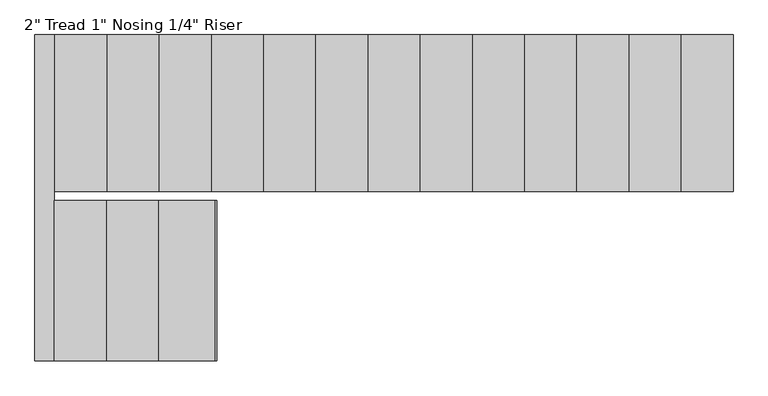
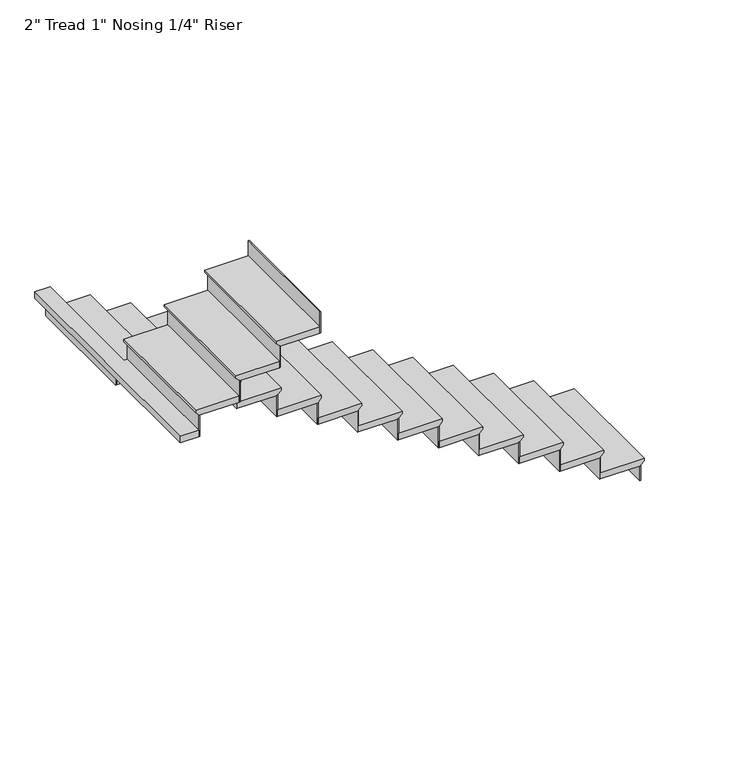
"""IFC4 building model written with IfcOpenShell, lengths in millimetres: stair flight geometry."""

from ifc_helpers import new_model, si_unit, origin, place, context, project, spatial, faceted_brep, source, transform, mapped, element, save


def stair_flight_dace13c7(model_context):
    return source(origin(), model_context, "Body", "Brep", [
        faceted_brep([(6794.5, 11386.0372886, 3198.2833333), (6794.5, 11386.0372886, 3217.3333333), (6794.5, 10471.6372886, 3217.3333333), (6794.5, 10471.6372886, 3198.2833333), (6769.1, 11386.0372886, 3172.8833333), (6769.1, 10471.6372886, 3172.8833333), (6464.3, 11386.0372886, 3217.3333333), (6464.3, 10471.6372886, 3217.3333333), (6769.1, 10471.6372886, 3166.5333333), (6464.3, 10471.6372886, 3166.5333333), (6464.3, 11386.0372886, 3166.5333333), (6769.1, 11386.0372886, 3166.5333333)], [[[0, 1, 2, 3]], [[4, 0, 3, 5]], [[2, 1, 6, 7]], [[8, 9, 10, 11]], [[2, 7, 9, 8, 5, 3]], [[8, 11, 4, 5]], [[6, 1, 0, 4, 11, 10]], [[7, 6, 10, 9]]]),
        faceted_brep([(6769.1, 11386.0372886, 3166.5333333), (6769.1, 11386.0372886, 3048.0), (6762.75, 11386.0372886, 3048.0), (6762.75, 11386.0372886, 3166.5333333), (6769.1, 10471.6372886, 3166.5333333), (6762.75, 10471.6372886, 3166.5333333), (6762.75, 10471.6372886, 3048.0), (6769.1, 10471.6372886, 3048.0)], [[[0, 1, 2, 3]], [[4, 5, 6, 7]], [[1, 0, 4, 7]], [[2, 1, 7, 6]], [[3, 2, 6, 5]], [[0, 3, 5, 4]]]),
        faceted_brep([(6464.3, 11386.0372886, 3335.8666667), (6464.3, 11386.0372886, 3166.5333333), (6457.95, 11386.0372886, 3166.5333333), (6457.95, 11386.0372886, 3335.8666667), (6464.3, 10471.6372886, 3335.8666667), (6457.95, 10471.6372886, 3335.8666667), (6457.95, 10471.6372886, 3166.5333333), (6464.3, 10471.6372886, 3166.5333333)], [[[0, 1, 2, 3]], [[4, 5, 6, 7]], [[1, 0, 4, 7]], [[2, 1, 7, 6]], [[3, 2, 6, 5]], [[0, 3, 5, 4]]]),
        faceted_brep([(6489.7, 10471.6372886, 3386.6666667), (6489.7, 11386.0372886, 3386.6666667), (6159.5, 11386.0372886, 3386.6666667), (6159.5, 10471.6372886, 3386.6666667), (6464.3, 10471.6372886, 3335.8666667), (6159.5, 10471.6372886, 3335.8666667), (6159.5, 11386.0372886, 3335.8666667), (6464.3, 11386.0372886, 3335.8666667), (6464.3, 10471.6372886, 3342.2166667), (6489.7, 10471.6372886, 3367.6166667), (6464.3, 11386.0372886, 3342.2166667), (6489.7, 11386.0372886, 3367.6166667)], [[[0, 1, 2, 3]], [[4, 5, 6, 7]], [[0, 3, 5, 4, 8, 9]], [[4, 7, 10, 8]], [[2, 1, 11, 10, 7, 6]], [[3, 2, 6, 5]], [[11, 1, 0, 9]], [[10, 11, 9, 8]]]),
        faceted_brep([(6159.5, 11386.0372886, 3505.2), (6159.5, 11386.0372886, 3335.8666667), (6153.15, 11386.0372886, 3335.8666667), (6153.15, 11386.0372886, 3505.2), (6159.5, 10471.6372886, 3505.2), (6153.15, 10471.6372886, 3505.2), (6153.15, 10471.6372886, 3335.8666667), (6159.5, 10471.6372886, 3335.8666667)], [[[0, 1, 2, 3]], [[4, 5, 6, 7]], [[1, 0, 4, 7]], [[2, 1, 7, 6]], [[3, 2, 6, 5]], [[0, 3, 5, 4]]]),
        faceted_brep([(6184.9, 10471.6372886, 3556.0), (6184.9, 11386.0372886, 3556.0), (5854.7, 11386.0372886, 3556.0), (5854.7, 10471.6372886, 3556.0), (6159.5, 10471.6372886, 3505.2), (5854.7, 10471.6372886, 3505.2), (5854.7, 11386.0372886, 3505.2), (6159.5, 11386.0372886, 3505.2), (6159.5, 10471.6372886, 3511.55), (6184.9, 10471.6372886, 3536.95), (6159.5, 11386.0372886, 3511.55), (6184.9, 11386.0372886, 3536.95)], [[[0, 1, 2, 3]], [[4, 5, 6, 7]], [[0, 3, 5, 4, 8, 9]], [[4, 7, 10, 8]], [[2, 1, 11, 10, 7, 6]], [[3, 2, 6, 5]], [[11, 1, 0, 9]], [[10, 11, 9, 8]]]),
        faceted_brep([(5854.7, 11386.0372886, 3674.5333333), (5854.7, 11386.0372886, 3505.2), (5848.35, 11386.0372886, 3505.2), (5848.35, 11386.0372886, 3674.5333333), (5854.7, 10471.6372886, 3674.5333333), (5848.35, 10471.6372886, 3674.5333333), (5848.35, 10471.6372886, 3505.2), (5854.7, 10471.6372886, 3505.2)], [[[0, 1, 2, 3]], [[4, 5, 6, 7]], [[1, 0, 4, 7]], [[2, 1, 7, 6]], [[3, 2, 6, 5]], [[0, 3, 5, 4]]]),
        faceted_brep([(5880.1, 10471.6372886, 3725.3333333), (5880.1, 11386.0372886, 3725.3333333), (5549.9, 11386.0372886, 3725.3333333), (5549.9, 10471.6372886, 3725.3333333), (5854.7, 10471.6372886, 3674.5333333), (5549.9, 10471.6372886, 3674.5333333), (5549.9, 11386.0372886, 3674.5333333), (5854.7, 11386.0372886, 3674.5333333), (5854.7, 10471.6372886, 3680.8833333), (5880.1, 10471.6372886, 3706.2833333), (5854.7, 11386.0372886, 3680.8833333), (5880.1, 11386.0372886, 3706.2833333)], [[[0, 1, 2, 3]], [[4, 5, 6, 7]], [[0, 3, 5, 4, 8, 9]], [[4, 7, 10, 8]], [[2, 1, 11, 10, 7, 6]], [[3, 2, 6, 5]], [[11, 1, 0, 9]], [[10, 11, 9, 8]]]),
        faceted_brep([(5549.9, 11386.0372886, 3843.8666667), (5549.9, 11386.0372886, 3674.5333333), (5543.55, 11386.0372886, 3674.5333333), (5543.55, 11386.0372886, 3843.8666667), (5549.9, 10471.6372886, 3843.8666667), (5543.55, 10471.6372886, 3843.8666667), (5543.55, 10471.6372886, 3674.5333333), (5549.9, 10471.6372886, 3674.5333333)], [[[0, 1, 2, 3]], [[4, 5, 6, 7]], [[1, 0, 4, 7]], [[2, 1, 7, 6]], [[3, 2, 6, 5]], [[0, 3, 5, 4]]]),
        faceted_brep([(5575.3, 10471.6372886, 3894.6666667), (5575.3, 11386.0372886, 3894.6666667), (5245.1, 11386.0372886, 3894.6666667), (5245.1, 10471.6372886, 3894.6666667), (5549.9, 10471.6372886, 3843.8666667), (5245.1, 10471.6372886, 3843.8666667), (5245.1, 11386.0372886, 3843.8666667), (5549.9, 11386.0372886, 3843.8666667), (5549.9, 10471.6372886, 3850.2166667), (5575.3, 10471.6372886, 3875.6166667), (5549.9, 11386.0372886, 3850.2166667), (5575.3, 11386.0372886, 3875.6166667)], [[[0, 1, 2, 3]], [[4, 5, 6, 7]], [[0, 3, 5, 4, 8, 9]], [[4, 7, 10, 8]], [[2, 1, 11, 10, 7, 6]], [[3, 2, 6, 5]], [[11, 1, 0, 9]], [[10, 11, 9, 8]]]),
        faceted_brep([(5245.1, 11386.0372886, 4013.2), (5245.1, 11386.0372886, 3843.8666667), (5238.75, 11386.0372886, 3843.8666667), (5238.75, 11386.0372886, 4013.2), (5245.1, 10471.6372886, 4013.2), (5238.75, 10471.6372886, 4013.2), (5238.75, 10471.6372886, 3843.8666667), (5245.1, 10471.6372886, 3843.8666667)], [[[0, 1, 2, 3]], [[4, 5, 6, 7]], [[1, 0, 4, 7]], [[2, 1, 7, 6]], [[3, 2, 6, 5]], [[0, 3, 5, 4]]]),
        faceted_brep([(5270.5, 10471.6372886, 4064.0), (5270.5, 11386.0372886, 4064.0), (4940.3, 11386.0372886, 4064.0), (4940.3, 10471.6372886, 4064.0), (5245.1, 10471.6372886, 4013.2), (4940.3, 10471.6372886, 4013.2), (4940.3, 11386.0372886, 4013.2), (5245.1, 11386.0372886, 4013.2), (5245.1, 10471.6372886, 4019.55), (5270.5, 10471.6372886, 4044.95), (5245.1, 11386.0372886, 4019.55), (5270.5, 11386.0372886, 4044.95)], [[[0, 1, 2, 3]], [[4, 5, 6, 7]], [[0, 3, 5, 4, 8, 9]], [[4, 7, 10, 8]], [[2, 1, 11, 10, 7, 6]], [[3, 2, 6, 5]], [[11, 1, 0, 9]], [[10, 11, 9, 8]]]),
        faceted_brep([(4940.3, 11386.0372886, 4182.5333333), (4940.3, 11386.0372886, 4013.2), (4933.95, 11386.0372886, 4013.2), (4933.95, 11386.0372886, 4182.5333333), (4940.3, 10471.6372886, 4182.5333333), (4933.95, 10471.6372886, 4182.5333333), (4933.95, 10471.6372886, 4013.2), (4940.3, 10471.6372886, 4013.2)], [[[0, 1, 2, 3]], [[4, 5, 6, 7]], [[1, 0, 4, 7]], [[2, 1, 7, 6]], [[3, 2, 6, 5]], [[0, 3, 5, 4]]]),
        faceted_brep([(4965.7, 10471.6372886, 4233.3333333), (4965.7, 11386.0372886, 4233.3333333), (4635.5, 11386.0372886, 4233.3333333), (4635.5, 10471.6372886, 4233.3333333), (4940.3, 10471.6372886, 4182.5333333), (4635.5, 10471.6372886, 4182.5333333), (4635.5, 11386.0372886, 4182.5333333), (4940.3, 11386.0372886, 4182.5333333), (4940.3, 10471.6372886, 4188.8833333), (4965.7, 10471.6372886, 4214.2833333), (4940.3, 11386.0372886, 4188.8833333), (4965.7, 11386.0372886, 4214.2833333)], [[[0, 1, 2, 3]], [[4, 5, 6, 7]], [[0, 3, 5, 4, 8, 9]], [[4, 7, 10, 8]], [[2, 1, 11, 10, 7, 6]], [[3, 2, 6, 5]], [[11, 1, 0, 9]], [[10, 11, 9, 8]]]),
        faceted_brep([(4635.5, 11386.0372886, 4351.8666667), (4635.5, 11386.0372886, 4182.5333333), (4629.15, 11386.0372886, 4182.5333333), (4629.15, 11386.0372886, 4351.8666667), (4635.5, 10471.6372886, 4351.8666667), (4629.15, 10471.6372886, 4351.8666667), (4629.15, 10471.6372886, 4182.5333333), (4635.5, 10471.6372886, 4182.5333333)], [[[0, 1, 2, 3]], [[4, 5, 6, 7]], [[1, 0, 4, 7]], [[2, 1, 7, 6]], [[3, 2, 6, 5]], [[0, 3, 5, 4]]]),
        faceted_brep([(4660.9, 10471.6372886, 4402.6666667), (4660.9, 11386.0372886, 4402.6666667), (4330.7, 11386.0372886, 4402.6666667), (4330.7, 10471.6372886, 4402.6666667), (4635.5, 10471.6372886, 4351.8666667), (4330.7, 10471.6372886, 4351.8666667), (4330.7, 11386.0372886, 4351.8666667), (4635.5, 11386.0372886, 4351.8666667), (4635.5, 10471.6372886, 4358.2166667), (4660.9, 10471.6372886, 4383.6166667), (4635.5, 11386.0372886, 4358.2166667), (4660.9, 11386.0372886, 4383.6166667)], [[[0, 1, 2, 3]], [[4, 5, 6, 7]], [[0, 3, 5, 4, 8, 9]], [[4, 7, 10, 8]], [[2, 1, 11, 10, 7, 6]], [[3, 2, 6, 5]], [[11, 1, 0, 9]], [[10, 11, 9, 8]]]),
        faceted_brep([(4330.7, 11386.0372886, 4521.2), (4330.7, 11386.0372886, 4351.8666667), (4324.35, 11386.0372886, 4351.8666667), (4324.35, 11386.0372886, 4521.2), (4330.7, 10471.6372886, 4521.2), (4324.35, 10471.6372886, 4521.2), (4324.35, 10471.6372886, 4351.8666667), (4330.7, 10471.6372886, 4351.8666667)], [[[0, 1, 2, 3]], [[4, 5, 6, 7]], [[1, 0, 4, 7]], [[2, 1, 7, 6]], [[3, 2, 6, 5]], [[0, 3, 5, 4]]]),
        faceted_brep([(4356.1, 10471.6372886, 4572.0), (4356.1, 11386.0372886, 4572.0), (4025.9, 11386.0372886, 4572.0), (4025.9, 10471.6372886, 4572.0), (4330.7, 10471.6372886, 4521.2), (4025.9, 10471.6372886, 4521.2), (4025.9, 11386.0372886, 4521.2), (4330.7, 11386.0372886, 4521.2), (4330.7, 10471.6372886, 4527.55), (4356.1, 10471.6372886, 4552.95), (4330.7, 11386.0372886, 4527.55), (4356.1, 11386.0372886, 4552.95)], [[[0, 1, 2, 3]], [[4, 5, 6, 7]], [[0, 3, 5, 4, 8, 9]], [[4, 7, 10, 8]], [[2, 1, 11, 10, 7, 6]], [[3, 2, 6, 5]], [[11, 1, 0, 9]], [[10, 11, 9, 8]]]),
        faceted_brep([(4025.9, 11386.0372886, 4690.5333333), (4025.9, 11386.0372886, 4521.2), (4019.55, 11386.0372886, 4521.2), (4019.55, 11386.0372886, 4690.5333333), (4025.9, 10471.6372886, 4690.5333333), (4019.55, 10471.6372886, 4690.5333333), (4019.55, 10471.6372886, 4521.2), (4025.9, 10471.6372886, 4521.2)], [[[0, 1, 2, 3]], [[4, 5, 6, 7]], [[1, 0, 4, 7]], [[2, 1, 7, 6]], [[3, 2, 6, 5]], [[0, 3, 5, 4]]]),
        faceted_brep([(4051.3, 10471.6372886, 4741.3333333), (4051.3, 11386.0372886, 4741.3333333), (3721.1, 11386.0372886, 4741.3333333), (3721.1, 10471.6372886, 4741.3333333), (4025.9, 10471.6372886, 4690.5333333), (3721.1, 10471.6372886, 4690.5333333), (3721.1, 11386.0372886, 4690.5333333), (4025.9, 11386.0372886, 4690.5333333), (4025.9, 10471.6372886, 4696.8833333), (4051.3, 10471.6372886, 4722.2833333), (4025.9, 11386.0372886, 4696.8833333), (4051.3, 11386.0372886, 4722.2833333)], [[[0, 1, 2, 3]], [[4, 5, 6, 7]], [[0, 3, 5, 4, 8, 9]], [[4, 7, 10, 8]], [[2, 1, 11, 10, 7, 6]], [[3, 2, 6, 5]], [[11, 1, 0, 9]], [[10, 11, 9, 8]]]),
        faceted_brep([(3721.1, 11386.0372886, 4859.8666667), (3721.1, 11386.0372886, 4690.5333333), (3714.75, 11386.0372886, 4690.5333333), (3714.75, 11386.0372886, 4859.8666667), (3721.1, 10471.6372886, 4859.8666667), (3714.75, 10471.6372886, 4859.8666667), (3714.75, 10471.6372886, 4690.5333333), (3721.1, 10471.6372886, 4690.5333333)], [[[0, 1, 2, 3]], [[4, 5, 6, 7]], [[1, 0, 4, 7]], [[2, 1, 7, 6]], [[3, 2, 6, 5]], [[0, 3, 5, 4]]]),
        faceted_brep([(3746.5, 10471.6372886, 4910.6666667), (3746.5, 11386.0372886, 4910.6666667), (3416.3, 11386.0372886, 4910.6666667), (3416.3, 10471.6372886, 4910.6666667), (3721.1, 10471.6372886, 4859.8666667), (3416.3, 10471.6372886, 4859.8666667), (3416.3, 11386.0372886, 4859.8666667), (3721.1, 11386.0372886, 4859.8666667), (3721.1, 10471.6372886, 4866.2166667), (3746.5, 10471.6372886, 4891.6166667), (3721.1, 11386.0372886, 4866.2166667), (3746.5, 11386.0372886, 4891.6166667)], [[[0, 1, 2, 3]], [[4, 5, 6, 7]], [[0, 3, 5, 4, 8, 9]], [[4, 7, 10, 8]], [[2, 1, 11, 10, 7, 6]], [[3, 2, 6, 5]], [[11, 1, 0, 9]], [[10, 11, 9, 8]]]),
        faceted_brep([(3416.3, 11386.0372886, 5029.2), (3416.3, 11386.0372886, 4859.8666667), (3409.95, 11386.0372886, 4859.8666667), (3409.95, 11386.0372886, 5029.2), (3416.3, 10471.6372886, 5029.2), (3409.95, 10471.6372886, 5029.2), (3409.95, 10471.6372886, 4859.8666667), (3416.3, 10471.6372886, 4859.8666667)], [[[0, 1, 2, 3]], [[4, 5, 6, 7]], [[1, 0, 4, 7]], [[2, 1, 7, 6]], [[3, 2, 6, 5]], [[0, 3, 5, 4]]]),
        faceted_brep([(3441.7, 10471.6372886, 5080.0), (3441.7, 11386.0372886, 5080.0), (3111.5, 11386.0372886, 5080.0), (3111.5, 10471.6372886, 5080.0), (3416.3, 10471.6372886, 5029.2), (3111.5, 10471.6372886, 5029.2), (3111.5, 11386.0372886, 5029.2), (3416.3, 11386.0372886, 5029.2), (3416.3, 10471.6372886, 5035.55), (3441.7, 10471.6372886, 5060.95), (3416.3, 11386.0372886, 5035.55), (3441.7, 11386.0372886, 5060.95)], [[[0, 1, 2, 3]], [[4, 5, 6, 7]], [[0, 3, 5, 4, 8, 9]], [[4, 7, 10, 8]], [[2, 1, 11, 10, 7, 6]], [[3, 2, 6, 5]], [[11, 1, 0, 9]], [[10, 11, 9, 8]]]),
        faceted_brep([(3111.5, 11386.0372886, 5198.5333333), (3111.5, 11386.0372886, 5029.2), (3105.15, 11386.0372886, 5029.2), (3105.15, 11386.0372886, 5198.5333333), (3111.5, 10471.6372886, 5198.5333333), (3105.15, 10471.6372886, 5198.5333333), (3105.15, 10471.6372886, 5029.2), (3111.5, 10471.6372886, 5029.2)], [[[0, 1, 2, 3]], [[4, 5, 6, 7]], [[1, 0, 4, 7]], [[2, 1, 7, 6]], [[3, 2, 6, 5]], [[0, 3, 5, 4]]]),
        faceted_brep([(3136.9, 10471.6372886, 5249.3333333), (3136.9, 11386.0372886, 5249.3333333), (2806.7, 11386.0372886, 5249.3333333), (2806.7, 10471.6372886, 5249.3333333), (3111.5, 10471.6372886, 5198.5333333), (2806.7, 10471.6372886, 5198.5333333), (2806.7, 11386.0372886, 5198.5333333), (3111.5, 11386.0372886, 5198.5333333), (3111.5, 10471.6372886, 5204.8833333), (3136.9, 10471.6372886, 5230.2833333), (3111.5, 11386.0372886, 5204.8833333), (3136.9, 11386.0372886, 5230.2833333)], [[[0, 1, 2, 3]], [[4, 5, 6, 7]], [[0, 3, 5, 4, 8, 9]], [[4, 7, 10, 8]], [[2, 1, 11, 10, 7, 6]], [[3, 2, 6, 5]], [[11, 1, 0, 9]], [[10, 11, 9, 8]]]),
        faceted_brep([(2806.7, 11386.0372886, 5367.8666667), (2806.7, 11386.0372886, 5198.5333333), (2800.35, 11386.0372886, 5198.5333333), (2800.35, 11386.0372886, 5367.8666667), (2806.7, 10471.6372886, 5367.8666667), (2800.35, 10471.6372886, 5367.8666667), (2800.35, 10471.6372886, 5198.5333333), (2806.7, 10471.6372886, 5198.5333333)], [[[0, 1, 2, 3]], [[4, 5, 6, 7]], [[1, 0, 4, 7]], [[2, 1, 7, 6]], [[3, 2, 6, 5]], [[0, 3, 5, 4]]]),
        faceted_brep([(2857.5, 10418.2972886, 5418.6666667), (2832.1, 10418.2972886, 5418.6666667), (2832.1, 11386.0372886, 5418.6666667), (2717.8, 11386.0372886, 5418.6666667), (2717.8, 9481.0372886, 5418.6666667), (2857.5, 9481.0372886, 5418.6666667), (2832.1, 10418.2972886, 5367.8666667), (2857.5, 10418.2972886, 5367.8666667), (2857.5, 9481.0372886, 5367.8666667), (2717.8, 9481.0372886, 5367.8666667), (2717.8, 11386.0372886, 5367.8666667), (2806.7, 11386.0372886, 5367.8666667), (2806.7, 10471.6372886, 5367.8666667), (2832.1, 10471.6372886, 5367.8666667), (2832.1, 10471.6372886, 5399.6166667), (2832.1, 11386.0372886, 5399.6166667), (2806.7, 10471.6372886, 5374.2166667), (2806.7, 11386.0372886, 5374.2166667)], [[[0, 1, 2, 3, 4, 5]], [[6, 7, 8, 9, 10, 11, 12, 13]], [[1, 0, 7, 6]], [[2, 1, 6, 13, 14, 15]], [[13, 12, 16, 14]], [[12, 11, 17, 16]], [[3, 2, 15, 17, 11, 10]], [[4, 3, 10, 9]], [[5, 4, 9, 8]], [[0, 5, 8, 7]], [[17, 15, 14, 16]]]),
        faceted_brep([(2857.5, 9481.0372886, 5537.2), (2857.5, 9481.0372886, 5367.8666667), (2863.85, 9481.0372886, 5367.8666667), (2863.85, 9481.0372886, 5537.2), (2857.5, 10418.2972886, 5537.2), (2863.85, 10418.2972886, 5537.2), (2863.85, 10418.2972886, 5367.8666667), (2857.5, 10418.2972886, 5367.8666667)], [[[0, 1, 2, 3]], [[4, 5, 6, 7]], [[1, 0, 4, 7]], [[2, 1, 7, 6]], [[3, 2, 6, 5]], [[0, 3, 5, 4]]]),
        faceted_brep([(2832.1, 10418.2972886, 5588.0), (2832.1, 9481.0372886, 5588.0), (3162.3, 9481.0372886, 5588.0), (3162.3, 10418.2972886, 5588.0), (2857.5, 10418.2972886, 5537.2), (3162.3, 10418.2972886, 5537.2), (3162.3, 9481.0372886, 5537.2), (2857.5, 9481.0372886, 5537.2), (2857.5, 10418.2972886, 5543.55), (2832.1, 10418.2972886, 5568.95), (2857.5, 9481.0372886, 5543.55), (2832.1, 9481.0372886, 5568.95)], [[[0, 1, 2, 3]], [[4, 5, 6, 7]], [[0, 3, 5, 4, 8, 9]], [[4, 7, 10, 8]], [[2, 1, 11, 10, 7, 6]], [[3, 2, 6, 5]], [[11, 1, 0, 9]], [[10, 11, 9, 8]]]),
        faceted_brep([(3162.3, 9481.0372886, 5706.5333333), (3162.3, 9481.0372886, 5537.2), (3168.65, 9481.0372886, 5537.2), (3168.65, 9481.0372886, 5706.5333333), (3162.3, 10418.2972886, 5706.5333333), (3168.65, 10418.2972886, 5706.5333333), (3168.65, 10418.2972886, 5537.2), (3162.3, 10418.2972886, 5537.2)], [[[0, 1, 2, 3]], [[4, 5, 6, 7]], [[1, 0, 4, 7]], [[2, 1, 7, 6]], [[3, 2, 6, 5]], [[0, 3, 5, 4]]]),
        faceted_brep([(3136.9, 10418.2972886, 5757.3333333), (3136.9, 9481.0372886, 5757.3333333), (3467.1, 9481.0372886, 5757.3333333), (3467.1, 10418.2972886, 5757.3333333), (3162.3, 10418.2972886, 5706.5333333), (3467.1, 10418.2972886, 5706.5333333), (3467.1, 9481.0372886, 5706.5333333), (3162.3, 9481.0372886, 5706.5333333), (3162.3, 10418.2972886, 5712.8833333), (3136.9, 10418.2972886, 5738.2833333), (3162.3, 9481.0372886, 5712.8833333), (3136.9, 9481.0372886, 5738.2833333)], [[[0, 1, 2, 3]], [[4, 5, 6, 7]], [[0, 3, 5, 4, 8, 9]], [[4, 7, 10, 8]], [[2, 1, 11, 10, 7, 6]], [[3, 2, 6, 5]], [[11, 1, 0, 9]], [[10, 11, 9, 8]]]),
        faceted_brep([(3467.1, 9481.0372886, 5875.8666667), (3467.1, 9481.0372886, 5706.5333333), (3473.45, 9481.0372886, 5706.5333333), (3473.45, 9481.0372886, 5875.8666667), (3467.1, 10418.2972886, 5875.8666667), (3473.45, 10418.2972886, 5875.8666667), (3473.45, 10418.2972886, 5706.5333333), (3467.1, 10418.2972886, 5706.5333333)], [[[0, 1, 2, 3]], [[4, 5, 6, 7]], [[1, 0, 4, 7]], [[2, 1, 7, 6]], [[3, 2, 6, 5]], [[0, 3, 5, 4]]]),
        faceted_brep([(3771.9019847, 9481.0372886, 6045.2), (3771.9019847, 9481.0372886, 5875.8666667), (3778.2519847, 9481.0372886, 5875.8666667), (3778.2519847, 9481.0372886, 6045.2), (3771.9019847, 10418.2972886, 6045.2), (3778.2519847, 10418.2972886, 6045.2), (3778.2519847, 10418.2972886, 5875.8666667), (3771.9019847, 10418.2972886, 5875.8666667)], [[[0, 1, 2, 3]], [[4, 5, 6, 7]], [[1, 0, 4, 7]], [[2, 1, 7, 6]], [[3, 2, 6, 5]], [[0, 3, 5, 4]]]),
        faceted_brep([(3441.7, 10418.2972886, 5926.6666667), (3441.7, 9481.0372886, 5926.6666667), (3771.9019847, 9481.0372886, 5926.6666667), (3771.9019847, 10418.2972886, 5926.6666667), (3467.1, 10418.2972886, 5875.8666667), (3771.9019847, 10418.2972886, 5875.8666667), (3771.9019847, 9481.0372886, 5875.8666667), (3467.1, 9481.0372886, 5875.8666667), (3467.1, 10418.2972886, 5882.2166667), (3441.7, 10418.2972886, 5907.6166667), (3467.1, 9481.0372886, 5882.2166667), (3441.7, 9481.0372886, 5907.6166667)], [[[0, 1, 2, 3]], [[4, 5, 6, 7]], [[0, 3, 5, 4, 8, 9]], [[4, 7, 10, 8]], [[2, 1, 11, 10, 7, 6]], [[3, 2, 6, 5]], [[11, 1, 0, 9]], [[10, 11, 9, 8]]]),
    ])


if __name__ == "__main__":
    model = new_model("IFC4")
    model_context = context("Model", 3, world=origin())
    ifc_project = project(units=[si_unit("LENGTHUNIT", "METRE", prefix="MILLI")], contexts=[model_context])
    site = spatial("IfcSite", under=ifc_project)
    building = spatial("IfcBuilding", under=site)
    placement = place(None, origin())
    stair_flight_shape = stair_flight_dace13c7(model_context)
    element("IfcStairFlight", 1, ObjectType="2\" Tread 1\" Nosing 1/4\" Riser", at=placement, inside=building, context=model_context, shape_type="MappedRepresentation", body=[
        mapped(stair_flight_shape, transform((0.0, 0.0, 0.0), x_axis=(1.0, 0.0, 0.0), y_axis=(0.0, 1.0, 0.0), z_axis=(0.0, 0.0, 1.0))),
    ])
    save(model, "model.ifc")
